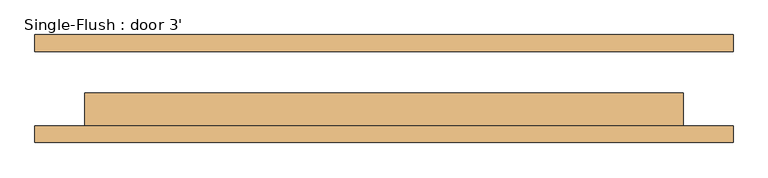
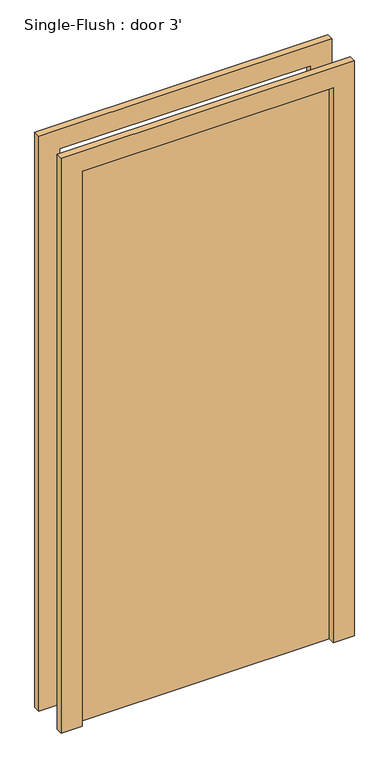
"""IFC4 building model written with IfcOpenShell, lengths in millimetres: door geometry, Single-Flush : door 3'."""

from ifc_helpers import new_model, si_unit, frame, origin, origin_with_axes, place, context, project, spatial, polyline, outline, extrude, source, transform, mapped, element, save


def single_flush_door_3_305aa2a5(model_context):
    return source(origin(), model_context, "Body", "SweptSolid", [
        extrude(outline(polyline([(2209.8, -533.4), (0.0, -533.4), (0.0, -457.2), (2133.6, -457.2), (2133.6, 457.2), (0.0, 457.2), (0.0, 533.4), (2209.8, 533.4), (2209.8, -533.4)])), frame((0.0, -82.55, 0.0), z_axis=(0.0, 1.0, 0.0), x_axis=(0.0, 0.0, 1.0)), (0.0, 0.0, 1.0), 25.4),
        extrude(outline(polyline([(2209.8, 533.4), (2209.8, -533.4), (0.0, -533.4), (0.0, -457.2), (2133.6, -457.2), (2133.6, 457.2), (0.0, 457.2), (0.0, 533.4), (2209.8, 533.4)])), frame((0.0, 57.15, 0.0), z_axis=(0.0, 1.0, 0.0), x_axis=(0.0, 0.0, 1.0)), (0.0, 0.0, 1.0), 25.4),
        extrude(outline(polyline([(457.2, -6.35), (457.2, -57.15), (-457.2, -57.15), (-457.2, -6.35), (457.2, -6.35)])), origin_with_axes(), (0.0, 0.0, 1.0), 2133.6),
    ])


if __name__ == "__main__":
    model = new_model("IFC4")
    model_context = context("Model", 3, world=origin())
    ifc_project = project(units=[si_unit("LENGTHUNIT", "METRE", prefix="MILLI")], contexts=[model_context])
    site = spatial("IfcSite", under=ifc_project)
    building = spatial("IfcBuilding", under=site)
    placement = place(None, origin())
    single_flush_door_3_shape = single_flush_door_3_305aa2a5(model_context)
    element("IfcDoor", 1, ObjectType="Single-Flush : door 3'", at=placement, inside=building, context=model_context, shape_type="MappedRepresentation", body=[
        mapped(single_flush_door_3_shape, transform((0.0, 0.0, 0.0), x_axis=(1.0, 0.0, 0.0), y_axis=(0.0, 1.0, 0.0), z_axis=(0.0, 0.0, 1.0))),
    ])
    save(model, "model.ifc")

# Revit data of these elements
# Type "Single-Flush : door 3'"
#   Type Mark = "8"
#   Construction Type Id = "MDOOR"
#   Assembly Code = "C1020"
#   Analytic Construction = "Metal"
#   Thickness = 0' - 2"
#   Heat Transfer Coefficient (U) = 0.651978 BTU/(h·ft²·°F)
#   Height = 7' - 0"
#   Trim Projection Ext = 0' - 1"
#   Trim Projection Int = 0' - 1"
#   Trim Width = 0' - 3"
#   Width = 3' - 0"
#   Define Thermal Properties by = 1
#   Door Material = Door - Panel
#   Frame Material = Door - Frame
#   Visual Light Transmittance = 0
#   Solar Heat Gain Coefficient = 0
#   Function = (empty or 0)
#   Wall Closure = (empty or 0)
# Element 1 (IfcDoor, "Single-Flush : door 3'")
#   Materials on its faces: "Door - Frame", "Door - Panel"
# Materials
#   "Door - Panel": class "Wood", colour RGB 210 159 95, transparency 0, Cost = 0
#   "Door - Frame": colour RGB 118 70 51, transparency 0, Cost = 0
